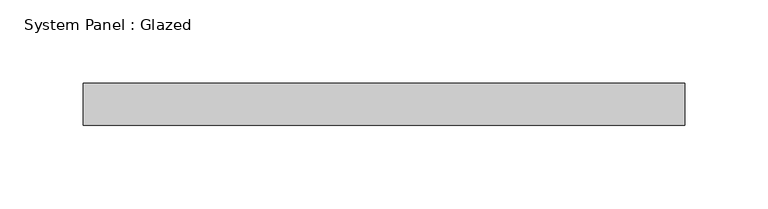
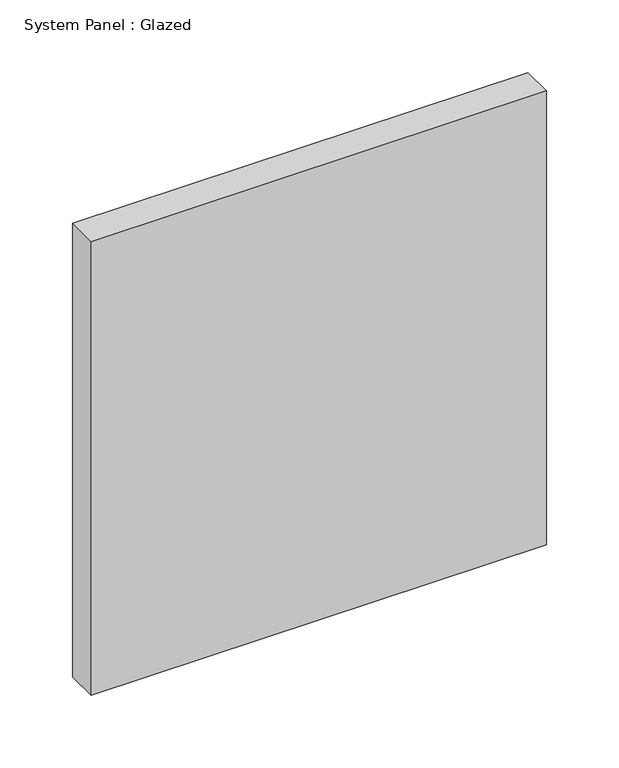
"""IFC4 building model written with IfcOpenShell, lengths in millimetres: plate geometry, System Panel : Glazed."""

from ifc_helpers import new_model, si_unit, origin, origin_with_axes, place, context, project, spatial, polyline, outline, extrude, source, transform, mapped, element, save


def system_panel_glazed_5d34ab6a(model_context):
    return source(origin(), model_context, "Body", "SweptSolid", [
        extrude(outline(polyline([(180.975, 19.05), (-180.975, 19.05), (-180.975, 44.45), (180.975, 44.45), (180.975, 19.05)])), origin_with_axes(), (0.0, 0.0, 1.0), 381.0),
    ])


if __name__ == "__main__":
    model = new_model("IFC4")
    model_context = context("Model", 3, world=origin())
    ifc_project = project(units=[si_unit("LENGTHUNIT", "METRE", prefix="MILLI")], contexts=[model_context])
    site = spatial("IfcSite", under=ifc_project)
    building = spatial("IfcBuilding", under=site)
    placement = place(None, origin())
    system_panel_glazed_shape = system_panel_glazed_5d34ab6a(model_context)
    element("IfcPlate", 1, ObjectType="System Panel : Glazed", at=placement, inside=building, context=model_context, shape_type="MappedRepresentation", body=[
        mapped(system_panel_glazed_shape, transform((0.0, 0.0, 0.0), x_axis=(1.0, 0.0, 0.0), y_axis=(0.0, 1.0, 0.0), z_axis=(0.0, 0.0, 1.0))),
    ])
    save(model, "model.ifc")

# Revit data of these elements
# Type "System Panel : Glazed"
#   Construction Type Id = "GSP4R"
#   Analytic Construction = "1/8 in Pilkington single glazing"
#   Visual Light Transmittance = 0.9
#   Solar Heat Gain Coefficient = 0.86
#   Heat Transfer Coefficient (U) = 1.18115 BTU/(h·ft²·°F)
#   Define Thermal Properties by = 1
# Element 1 (IfcPlate, "System Panel : Glazed")
#   Materials on its faces: "Glass"
# Materials
#   "Glass": class "Glass", colour RGB 0 128 192, transparency 0.75, Description = "Soda Lime Glass", Cost = 0
